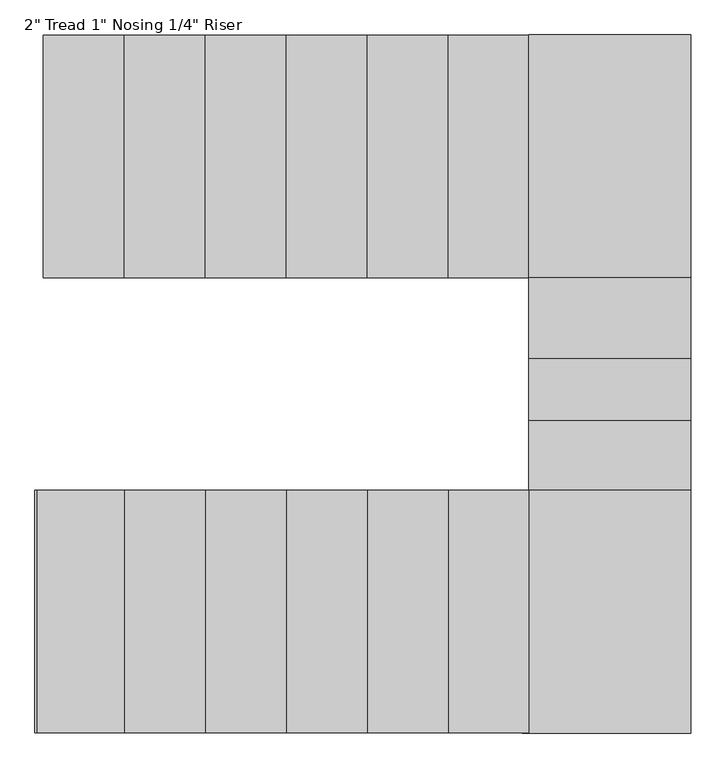
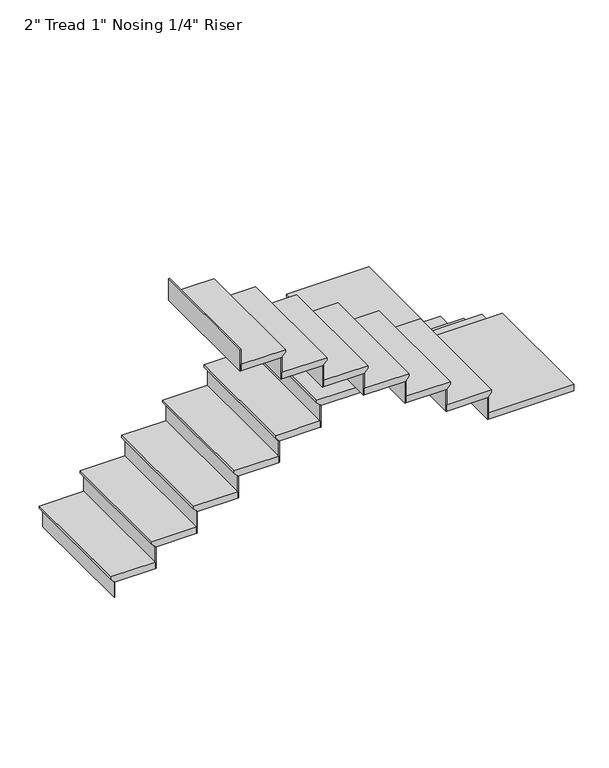
"""IFC4 building model written with IfcOpenShell, lengths in millimetres: stair flight geometry."""

from ifc_helpers import new_model, si_unit, origin, place, context, project, spatial, faceted_brep, source, transform, mapped, element, save


def stair_flight_95d2f6bb(model_context):
    return source(origin(), model_context, "Body", "Brep", [
        faceted_brep([(6477.0, 10054.8323212, 6246.2833333), (6477.0, 10054.8323212, 6265.3333333), (6477.0, 10969.2323212, 6265.3333333), (6477.0, 10969.2323212, 6246.2833333), (6502.4, 10054.8323212, 6220.8833333), (6502.4, 10969.2323212, 6220.8833333), (6807.2, 10054.8323212, 6265.3333333), (6807.2, 10969.2323212, 6265.3333333), (6502.4, 10969.2323212, 6214.5333333), (6807.2, 10969.2323212, 6214.5333333), (6807.2, 10054.8323212, 6214.5333333), (6502.4, 10054.8323212, 6214.5333333)], [[[0, 1, 2, 3]], [[4, 0, 3, 5]], [[2, 1, 6, 7]], [[8, 9, 10, 11]], [[2, 7, 9, 8, 5, 3]], [[8, 11, 4, 5]], [[6, 1, 0, 4, 11, 10]], [[7, 6, 10, 9]]]),
        faceted_brep([(6502.4, 10054.8323212, 6214.5333333), (6502.4, 10054.8323212, 6096.0), (6508.75, 10054.8323212, 6096.0), (6508.75, 10054.8323212, 6214.5333333), (6502.4, 10969.2323212, 6214.5333333), (6508.75, 10969.2323212, 6214.5333333), (6508.75, 10969.2323212, 6096.0), (6502.4, 10969.2323212, 6096.0)], [[[0, 1, 2, 3]], [[4, 5, 6, 7]], [[1, 0, 4, 7]], [[2, 1, 7, 6]], [[3, 2, 6, 5]], [[0, 3, 5, 4]]]),
        faceted_brep([(6807.2, 10054.8323212, 6383.8666667), (6807.2, 10054.8323212, 6214.5333333), (6813.55, 10054.8323212, 6214.5333333), (6813.55, 10054.8323212, 6383.8666667), (6807.2, 10969.2323212, 6383.8666667), (6813.55, 10969.2323212, 6383.8666667), (6813.55, 10969.2323212, 6214.5333333), (6807.2, 10969.2323212, 6214.5333333)], [[[0, 1, 2, 3]], [[4, 5, 6, 7]], [[1, 0, 4, 7]], [[2, 1, 7, 6]], [[3, 2, 6, 5]], [[0, 3, 5, 4]]]),
        faceted_brep([(6781.8, 10969.2323212, 6434.6666667), (6781.8, 10054.8323212, 6434.6666667), (7112.0, 10054.8323212, 6434.6666667), (7112.0, 10969.2323212, 6434.6666667), (6807.2, 10969.2323212, 6383.8666667), (7112.0, 10969.2323212, 6383.8666667), (7112.0, 10054.8323212, 6383.8666667), (6807.2, 10054.8323212, 6383.8666667), (6807.2, 10969.2323212, 6390.2166667), (6781.8, 10969.2323212, 6415.6166667), (6807.2, 10054.8323212, 6390.2166667), (6781.8, 10054.8323212, 6415.6166667)], [[[0, 1, 2, 3]], [[4, 5, 6, 7]], [[0, 3, 5, 4, 8, 9]], [[4, 7, 10, 8]], [[2, 1, 11, 10, 7, 6]], [[3, 2, 6, 5]], [[11, 1, 0, 9]], [[10, 11, 9, 8]]]),
        faceted_brep([(7112.0, 10054.8323212, 6553.2), (7112.0, 10054.8323212, 6383.8666667), (7118.35, 10054.8323212, 6383.8666667), (7118.35, 10054.8323212, 6553.2), (7112.0, 10969.2323212, 6553.2), (7118.35, 10969.2323212, 6553.2), (7118.35, 10969.2323212, 6383.8666667), (7112.0, 10969.2323212, 6383.8666667)], [[[0, 1, 2, 3]], [[4, 5, 6, 7]], [[1, 0, 4, 7]], [[2, 1, 7, 6]], [[3, 2, 6, 5]], [[0, 3, 5, 4]]]),
        faceted_brep([(7086.6, 10969.2323212, 6604.0), (7086.6, 10054.8323212, 6604.0), (7416.8, 10054.8323212, 6604.0), (7416.8, 10969.2323212, 6604.0), (7112.0, 10969.2323212, 6553.2), (7416.8, 10969.2323212, 6553.2), (7416.8, 10054.8323212, 6553.2), (7112.0, 10054.8323212, 6553.2), (7112.0, 10969.2323212, 6559.55), (7086.6, 10969.2323212, 6584.95), (7112.0, 10054.8323212, 6559.55), (7086.6, 10054.8323212, 6584.95)], [[[0, 1, 2, 3]], [[4, 5, 6, 7]], [[0, 3, 5, 4, 8, 9]], [[4, 7, 10, 8]], [[2, 1, 11, 10, 7, 6]], [[3, 2, 6, 5]], [[11, 1, 0, 9]], [[10, 11, 9, 8]]]),
        faceted_brep([(7416.8, 10054.8323212, 6722.5333333), (7416.8, 10054.8323212, 6553.2), (7423.15, 10054.8323212, 6553.2), (7423.15, 10054.8323212, 6722.5333333), (7416.8, 10969.2323212, 6722.5333333), (7423.15, 10969.2323212, 6722.5333333), (7423.15, 10969.2323212, 6553.2), (7416.8, 10969.2323212, 6553.2)], [[[0, 1, 2, 3]], [[4, 5, 6, 7]], [[1, 0, 4, 7]], [[2, 1, 7, 6]], [[3, 2, 6, 5]], [[0, 3, 5, 4]]]),
        faceted_brep([(7391.4, 10969.2323212, 6773.3333333), (7391.4, 10054.8323212, 6773.3333333), (7721.6, 10054.8323212, 6773.3333333), (7721.6, 10969.2323212, 6773.3333333), (7416.8, 10969.2323212, 6722.5333333), (7721.6, 10969.2323212, 6722.5333333), (7721.6, 10054.8323212, 6722.5333333), (7416.8, 10054.8323212, 6722.5333333), (7416.8, 10969.2323212, 6728.8833333), (7391.4, 10969.2323212, 6754.2833333), (7416.8, 10054.8323212, 6728.8833333), (7391.4, 10054.8323212, 6754.2833333)], [[[0, 1, 2, 3]], [[4, 5, 6, 7]], [[0, 3, 5, 4, 8, 9]], [[4, 7, 10, 8]], [[2, 1, 11, 10, 7, 6]], [[3, 2, 6, 5]], [[11, 1, 0, 9]], [[10, 11, 9, 8]]]),
        faceted_brep([(7721.6, 10054.8323212, 6891.8666667), (7721.6, 10054.8323212, 6722.5333333), (7727.95, 10054.8323212, 6722.5333333), (7727.95, 10054.8323212, 6891.8666667), (7721.6, 10969.2323212, 6891.8666667), (7727.95, 10969.2323212, 6891.8666667), (7727.95, 10969.2323212, 6722.5333333), (7721.6, 10969.2323212, 6722.5333333)], [[[0, 1, 2, 3]], [[4, 5, 6, 7]], [[1, 0, 4, 7]], [[2, 1, 7, 6]], [[3, 2, 6, 5]], [[0, 3, 5, 4]]]),
        faceted_brep([(7696.2, 10969.2323212, 6942.6666667), (7696.2, 10054.8323212, 6942.6666667), (8026.4, 10054.8323212, 6942.6666667), (8026.4, 10969.2323212, 6942.6666667), (7721.6, 10969.2323212, 6891.8666667), (8026.4, 10969.2323212, 6891.8666667), (8026.4, 10054.8323212, 6891.8666667), (7721.6, 10054.8323212, 6891.8666667), (7721.6, 10969.2323212, 6898.2166667), (7696.2, 10969.2323212, 6923.6166667), (7721.6, 10054.8323212, 6898.2166667), (7696.2, 10054.8323212, 6923.6166667)], [[[0, 1, 2, 3]], [[4, 5, 6, 7]], [[0, 3, 5, 4, 8, 9]], [[4, 7, 10, 8]], [[2, 1, 11, 10, 7, 6]], [[3, 2, 6, 5]], [[11, 1, 0, 9]], [[10, 11, 9, 8]]]),
        faceted_brep([(8026.4, 10054.8323212, 7061.2), (8026.4, 10054.8323212, 6891.8666667), (8032.75, 10054.8323212, 6891.8666667), (8032.75, 10054.8323212, 7061.2), (8026.4, 10969.2323212, 7061.2), (8032.75, 10969.2323212, 7061.2), (8032.75, 10969.2323212, 6891.8666667), (8026.4, 10969.2323212, 6891.8666667)], [[[0, 1, 2, 3]], [[4, 5, 6, 7]], [[1, 0, 4, 7]], [[2, 1, 7, 6]], [[3, 2, 6, 5]], [[0, 3, 5, 4]]]),
        faceted_brep([(8001.0, 10969.2323212, 7112.0), (8001.0, 10054.8323212, 7112.0), (8331.2, 10054.8323212, 7112.0), (8331.2, 10969.2323212, 7112.0), (8026.4, 10969.2323212, 7061.2), (8331.2, 10969.2323212, 7061.2), (8331.2, 10054.8323212, 7061.2), (8026.4, 10054.8323212, 7061.2), (8026.4, 10969.2323212, 7067.55), (8001.0, 10969.2323212, 7092.95), (8026.4, 10054.8323212, 7067.55), (8001.0, 10054.8323212, 7092.95)], [[[0, 1, 2, 3]], [[4, 5, 6, 7]], [[0, 3, 5, 4, 8, 9]], [[4, 7, 10, 8]], [[2, 1, 11, 10, 7, 6]], [[3, 2, 6, 5]], [[11, 1, 0, 9]], [[10, 11, 9, 8]]]),
        faceted_brep([(8331.2, 10054.8323212, 7230.5333333), (8331.2, 10054.8323212, 7061.2), (8337.55, 10054.8323212, 7061.2), (8337.55, 10054.8323212, 7230.5333333), (8331.2, 10969.2323212, 7230.5333333), (8337.55, 10969.2323212, 7230.5333333), (8337.55, 10969.2323212, 7061.2), (8331.2, 10969.2323212, 7061.2)], [[[0, 1, 2, 3]], [[4, 5, 6, 7]], [[1, 0, 4, 7]], [[2, 1, 7, 6]], [[3, 2, 6, 5]], [[0, 3, 5, 4]]]),
        faceted_brep([(8915.4, 10029.4323212, 7281.3333333), (8915.4, 10969.2323212, 7281.3333333), (8305.8, 10969.2323212, 7281.3333333), (8305.8, 10029.4323212, 7281.3333333), (8915.4, 10969.2323212, 7230.5333333), (8915.4, 10029.4323212, 7230.5333333), (8305.8, 10029.4323212, 7230.5333333), (8305.8, 10054.8323212, 7230.5333333), (8331.2, 10054.8323212, 7230.5333333), (8331.2, 10969.2323212, 7230.5333333), (8331.2, 10969.2323212, 7236.8833333), (8305.8, 10969.2323212, 7262.2833333), (8331.2, 10054.8323212, 7236.8833333), (8305.8, 10054.8323212, 7262.2833333)], [[[0, 1, 2, 3]], [[4, 5, 6, 7, 8, 9]], [[1, 0, 5, 4]], [[2, 1, 4, 9, 10, 11]], [[9, 8, 12, 10]], [[8, 7, 13, 12]], [[3, 2, 11, 13, 7, 6]], [[0, 3, 6, 5]], [[11, 10, 12, 13]]]),
        faceted_brep([(8305.8, 10029.4323212, 7399.8666667), (8305.8, 10029.4323212, 7230.5333333), (8305.8, 10023.0823212, 7230.5333333), (8305.8, 10023.0823212, 7399.8666667), (8915.4, 10029.4323212, 7399.8666667), (8915.4, 10023.0823212, 7399.8666667), (8915.4, 10023.0823212, 7230.5333333), (8915.4, 10029.4323212, 7230.5333333)], [[[0, 1, 2, 3]], [[4, 5, 6, 7]], [[1, 0, 4, 7]], [[2, 1, 7, 6]], [[3, 2, 6, 5]], [[0, 3, 5, 4]]]),
        faceted_brep([(8915.4, 10054.8323212, 7450.6666667), (8305.8, 10054.8323212, 7450.6666667), (8305.8, 9724.6323212, 7450.6666667), (8915.4, 9724.6323212, 7450.6666667), (8915.4, 10029.4323212, 7399.8666667), (8915.4, 9724.6323212, 7399.8666667), (8305.8, 9724.6323212, 7399.8666667), (8305.8, 10029.4323212, 7399.8666667), (8915.4, 10029.4323212, 7406.2166667), (8915.4, 10054.8323212, 7431.6166667), (8305.8, 10029.4323212, 7406.2166667), (8305.8, 10054.8323212, 7431.6166667)], [[[0, 1, 2, 3]], [[4, 5, 6, 7]], [[0, 3, 5, 4, 8, 9]], [[4, 7, 10, 8]], [[2, 1, 11, 10, 7, 6]], [[3, 2, 6, 5]], [[11, 1, 0, 9]], [[10, 11, 9, 8]]]),
        faceted_brep([(8305.8, 9724.6323212, 7569.2), (8305.8, 9724.6323212, 7399.8666667), (8305.8, 9718.2823212, 7399.8666667), (8305.8, 9718.2823212, 7569.2), (8915.4, 9724.6323212, 7569.2), (8915.4, 9718.2823212, 7569.2), (8915.4, 9718.2823212, 7399.8666667), (8915.4, 9724.6323212, 7399.8666667)], [[[0, 1, 2, 3]], [[4, 5, 6, 7]], [[1, 0, 4, 7]], [[2, 1, 7, 6]], [[3, 2, 6, 5]], [[0, 3, 5, 4]]]),
        faceted_brep([(8915.4, 9750.0323212, 7620.0), (8305.8, 9750.0323212, 7620.0), (8305.8, 9491.8832929, 7620.0), (8915.4, 9491.8832929, 7620.0), (8915.4, 9724.6323212, 7569.2), (8915.4, 9491.8832929, 7569.2), (8305.8, 9491.8832929, 7569.2), (8305.8, 9724.6323212, 7569.2), (8915.4, 9724.6323212, 7575.55), (8915.4, 9750.0323212, 7600.95), (8305.8, 9724.6323212, 7575.55), (8305.8, 9750.0323212, 7600.95)], [[[0, 1, 2, 3]], [[4, 5, 6, 7]], [[0, 3, 5, 4, 8, 9]], [[4, 7, 10, 8]], [[2, 1, 11, 10, 7, 6]], [[3, 2, 6, 5]], [[11, 1, 0, 9]], [[10, 11, 9, 8]]]),
        faceted_brep([(8305.8, 9491.8832929, 7738.5333333), (8305.8, 9491.8832929, 7569.2), (8305.8, 9485.5332929, 7569.2), (8305.8, 9485.5332929, 7738.5333333), (8915.4, 9491.8832929, 7738.5333333), (8915.4, 9485.5332929, 7738.5333333), (8915.4, 9485.5332929, 7569.2), (8915.4, 9491.8832929, 7569.2)], [[[0, 1, 2, 3]], [[4, 5, 6, 7]], [[1, 0, 4, 7]], [[2, 1, 7, 6]], [[3, 2, 6, 5]], [[0, 3, 5, 4]]]),
        faceted_brep([(8915.4, 9517.2832929, 7789.3333333), (8305.8, 9517.2832929, 7789.3333333), (8305.8, 9229.3323212, 7789.3333333), (8915.4, 9229.3323212, 7789.3333333), (8915.4, 9491.8832929, 7738.5333333), (8915.4, 9229.3323212, 7738.5333333), (8305.8, 9229.3323212, 7738.5333333), (8305.8, 9491.8832929, 7738.5333333), (8915.4, 9491.8832929, 7744.8833333), (8915.4, 9517.2832929, 7770.2833333), (8305.8, 9491.8832929, 7744.8833333), (8305.8, 9517.2832929, 7770.2833333)], [[[0, 1, 2, 3]], [[4, 5, 6, 7]], [[0, 3, 5, 4, 8, 9]], [[4, 7, 10, 8]], [[2, 1, 11, 10, 7, 6]], [[3, 2, 6, 5]], [[11, 1, 0, 9]], [[10, 11, 9, 8]]]),
        faceted_brep([(8305.8, 9229.3323212, 7907.8666667), (8305.8, 9229.3323212, 7738.5333333), (8305.8, 9222.9823212, 7738.5333333), (8305.8, 9222.9823212, 7907.8666667), (8915.4, 9229.3323212, 7907.8666667), (8915.4, 9222.9823212, 7907.8666667), (8915.4, 9222.9823212, 7738.5333333), (8915.4, 9229.3323212, 7738.5333333)], [[[0, 1, 2, 3]], [[4, 5, 6, 7]], [[1, 0, 4, 7]], [[2, 1, 7, 6]], [[3, 2, 6, 5]], [[0, 3, 5, 4]]]),
        faceted_brep([(8280.4, 8340.3323212, 7958.6666667), (8915.4, 8340.3323212, 7958.6666667), (8915.4, 9254.7323212, 7958.6666667), (8280.4, 9254.7323212, 7958.6666667), (8915.4, 8340.3323212, 7907.8666667), (8280.4, 8340.3323212, 7907.8666667), (8280.4, 9254.7323212, 7907.8666667), (8305.8, 9254.7323212, 7907.8666667), (8305.8, 9229.3323212, 7907.8666667), (8915.4, 9229.3323212, 7907.8666667), (8915.4, 9229.3323212, 7914.2166667), (8915.4, 9254.7323212, 7939.6166667), (8305.8, 9229.3323212, 7914.2166667), (8305.8, 9254.7323212, 7939.6166667)], [[[0, 1, 2, 3]], [[4, 5, 6, 7, 8, 9]], [[1, 0, 5, 4]], [[2, 1, 4, 9, 10, 11]], [[9, 8, 12, 10]], [[8, 7, 13, 12]], [[3, 2, 11, 13, 7, 6]], [[0, 3, 6, 5]], [[11, 10, 12, 13]]]),
        faceted_brep([(8280.4, 9254.7323212, 8077.2), (8280.4, 9254.7323212, 7907.8666667), (8274.05, 9254.7323212, 7907.8666667), (8274.05, 9254.7323212, 8077.2), (8280.4, 8340.3323212, 8077.2), (8274.05, 8340.3323212, 8077.2), (8274.05, 8340.3323212, 7907.8666667), (8280.4, 8340.3323212, 7907.8666667)], [[[0, 1, 2, 3]], [[4, 5, 6, 7]], [[1, 0, 4, 7]], [[2, 1, 7, 6]], [[3, 2, 6, 5]], [[0, 3, 5, 4]]]),
        faceted_brep([(8305.8, 8340.3323212, 8128.0), (8305.8, 9254.7323212, 8128.0), (7975.6, 9254.7323212, 8128.0), (7975.6, 8340.3323212, 8128.0), (8280.4, 8340.3323212, 8077.2), (7975.6, 8340.3323212, 8077.2), (7975.6, 9254.7323212, 8077.2), (8280.4, 9254.7323212, 8077.2), (8280.4, 8340.3323212, 8083.55), (8305.8, 8340.3323212, 8108.95), (8280.4, 9254.7323212, 8083.55), (8305.8, 9254.7323212, 8108.95)], [[[0, 1, 2, 3]], [[4, 5, 6, 7]], [[0, 3, 5, 4, 8, 9]], [[4, 7, 10, 8]], [[2, 1, 11, 10, 7, 6]], [[3, 2, 6, 5]], [[11, 1, 0, 9]], [[10, 11, 9, 8]]]),
        faceted_brep([(7975.6, 9254.7323212, 8246.5333333), (7975.6, 9254.7323212, 8077.2), (7969.25, 9254.7323212, 8077.2), (7969.25, 9254.7323212, 8246.5333333), (7975.6, 8340.3323212, 8246.5333333), (7969.25, 8340.3323212, 8246.5333333), (7969.25, 8340.3323212, 8077.2), (7975.6, 8340.3323212, 8077.2)], [[[0, 1, 2, 3]], [[4, 5, 6, 7]], [[1, 0, 4, 7]], [[2, 1, 7, 6]], [[3, 2, 6, 5]], [[0, 3, 5, 4]]]),
        faceted_brep([(8001.0, 8340.3323212, 8297.3333333), (8001.0, 9254.7323212, 8297.3333333), (7670.8, 9254.7323212, 8297.3333333), (7670.8, 8340.3323212, 8297.3333333), (7975.6, 8340.3323212, 8246.5333333), (7670.8, 8340.3323212, 8246.5333333), (7670.8, 9254.7323212, 8246.5333333), (7975.6, 9254.7323212, 8246.5333333), (7975.6, 8340.3323212, 8252.8833333), (8001.0, 8340.3323212, 8278.2833333), (7975.6, 9254.7323212, 8252.8833333), (8001.0, 9254.7323212, 8278.2833333)], [[[0, 1, 2, 3]], [[4, 5, 6, 7]], [[0, 3, 5, 4, 8, 9]], [[4, 7, 10, 8]], [[2, 1, 11, 10, 7, 6]], [[3, 2, 6, 5]], [[11, 1, 0, 9]], [[10, 11, 9, 8]]]),
        faceted_brep([(7670.8, 9254.7323212, 8415.8666667), (7670.8, 9254.7323212, 8246.5333333), (7664.45, 9254.7323212, 8246.5333333), (7664.45, 9254.7323212, 8415.8666667), (7670.8, 8340.3323212, 8415.8666667), (7664.45, 8340.3323212, 8415.8666667), (7664.45, 8340.3323212, 8246.5333333), (7670.8, 8340.3323212, 8246.5333333)], [[[0, 1, 2, 3]], [[4, 5, 6, 7]], [[1, 0, 4, 7]], [[2, 1, 7, 6]], [[3, 2, 6, 5]], [[0, 3, 5, 4]]]),
        faceted_brep([(7696.2, 8340.3323212, 8466.6666667), (7696.2, 9254.7323212, 8466.6666667), (7366.0, 9254.7323212, 8466.6666667), (7366.0, 8340.3323212, 8466.6666667), (7670.8, 8340.3323212, 8415.8666667), (7366.0, 8340.3323212, 8415.8666667), (7366.0, 9254.7323212, 8415.8666667), (7670.8, 9254.7323212, 8415.8666667), (7670.8, 8340.3323212, 8422.2166667), (7696.2, 8340.3323212, 8447.6166667), (7670.8, 9254.7323212, 8422.2166667), (7696.2, 9254.7323212, 8447.6166667)], [[[0, 1, 2, 3]], [[4, 5, 6, 7]], [[0, 3, 5, 4, 8, 9]], [[4, 7, 10, 8]], [[2, 1, 11, 10, 7, 6]], [[3, 2, 6, 5]], [[11, 1, 0, 9]], [[10, 11, 9, 8]]]),
        faceted_brep([(7366.0, 9254.7323212, 8585.2), (7366.0, 9254.7323212, 8415.8666667), (7359.65, 9254.7323212, 8415.8666667), (7359.65, 9254.7323212, 8585.2), (7366.0, 8340.3323212, 8585.2), (7359.65, 8340.3323212, 8585.2), (7359.65, 8340.3323212, 8415.8666667), (7366.0, 8340.3323212, 8415.8666667)], [[[0, 1, 2, 3]], [[4, 5, 6, 7]], [[1, 0, 4, 7]], [[2, 1, 7, 6]], [[3, 2, 6, 5]], [[0, 3, 5, 4]]]),
        faceted_brep([(7391.4, 8340.3323212, 8636.0), (7391.4, 9254.7323212, 8636.0), (7061.2, 9254.7323212, 8636.0), (7061.2, 8340.3323212, 8636.0), (7366.0, 8340.3323212, 8585.2), (7061.2, 8340.3323212, 8585.2), (7061.2, 9254.7323212, 8585.2), (7366.0, 9254.7323212, 8585.2), (7366.0, 8340.3323212, 8591.55), (7391.4, 8340.3323212, 8616.95), (7366.0, 9254.7323212, 8591.55), (7391.4, 9254.7323212, 8616.95)], [[[0, 1, 2, 3]], [[4, 5, 6, 7]], [[0, 3, 5, 4, 8, 9]], [[4, 7, 10, 8]], [[2, 1, 11, 10, 7, 6]], [[3, 2, 6, 5]], [[11, 1, 0, 9]], [[10, 11, 9, 8]]]),
        faceted_brep([(7061.2, 9254.7323212, 8754.5333333), (7061.2, 9254.7323212, 8585.2), (7054.85, 9254.7323212, 8585.2), (7054.85, 9254.7323212, 8754.5333333), (7061.2, 8340.3323212, 8754.5333333), (7054.85, 8340.3323212, 8754.5333333), (7054.85, 8340.3323212, 8585.2), (7061.2, 8340.3323212, 8585.2)], [[[0, 1, 2, 3]], [[4, 5, 6, 7]], [[1, 0, 4, 7]], [[2, 1, 7, 6]], [[3, 2, 6, 5]], [[0, 3, 5, 4]]]),
        faceted_brep([(7086.6, 8340.3323212, 8805.3333333), (7086.6, 9254.7323212, 8805.3333333), (6756.4, 9254.7323212, 8805.3333333), (6756.4, 8340.3323212, 8805.3333333), (7061.2, 8340.3323212, 8754.5333333), (6756.4, 8340.3323212, 8754.5333333), (6756.4, 9254.7323212, 8754.5333333), (7061.2, 9254.7323212, 8754.5333333), (7061.2, 8340.3323212, 8760.8833333), (7086.6, 8340.3323212, 8786.2833333), (7061.2, 9254.7323212, 8760.8833333), (7086.6, 9254.7323212, 8786.2833333)], [[[0, 1, 2, 3]], [[4, 5, 6, 7]], [[0, 3, 5, 4, 8, 9]], [[4, 7, 10, 8]], [[2, 1, 11, 10, 7, 6]], [[3, 2, 6, 5]], [[11, 1, 0, 9]], [[10, 11, 9, 8]]]),
        faceted_brep([(6756.4, 9254.7323212, 8923.8666667), (6756.4, 9254.7323212, 8754.5333333), (6750.05, 9254.7323212, 8754.5333333), (6750.05, 9254.7323212, 8923.8666667), (6756.4, 8340.3323212, 8923.8666667), (6750.05, 8340.3323212, 8923.8666667), (6750.05, 8340.3323212, 8754.5333333), (6756.4, 8340.3323212, 8754.5333333)], [[[0, 1, 2, 3]], [[4, 5, 6, 7]], [[1, 0, 4, 7]], [[2, 1, 7, 6]], [[3, 2, 6, 5]], [[0, 3, 5, 4]]]),
        faceted_brep([(6451.6, 9254.7323212, 9093.2), (6451.6, 9254.7323212, 8923.8666667), (6445.25, 9254.7323212, 8923.8666667), (6445.25, 9254.7323212, 9093.2), (6451.6, 8340.3323212, 9093.2), (6445.25, 8340.3323212, 9093.2), (6445.25, 8340.3323212, 8923.8666667), (6451.6, 8340.3323212, 8923.8666667)], [[[0, 1, 2, 3]], [[4, 5, 6, 7]], [[1, 0, 4, 7]], [[2, 1, 7, 6]], [[3, 2, 6, 5]], [[0, 3, 5, 4]]]),
        faceted_brep([(6781.8, 8340.3323212, 8974.6666667), (6781.8, 9254.7323212, 8974.6666667), (6451.6, 9254.7323212, 8974.6666667), (6451.6, 8340.3323212, 8974.6666667), (6756.4, 8340.3323212, 8923.8666667), (6451.6, 8340.3323212, 8923.8666667), (6451.6, 9254.7323212, 8923.8666667), (6756.4, 9254.7323212, 8923.8666667), (6756.4, 8340.3323212, 8930.2166667), (6781.8, 8340.3323212, 8955.6166667), (6756.4, 9254.7323212, 8930.2166667), (6781.8, 9254.7323212, 8955.6166667)], [[[0, 1, 2, 3]], [[4, 5, 6, 7]], [[0, 3, 5, 4, 8, 9]], [[4, 7, 10, 8]], [[2, 1, 11, 10, 7, 6]], [[3, 2, 6, 5]], [[11, 1, 0, 9]], [[10, 11, 9, 8]]]),
    ])


if __name__ == "__main__":
    model = new_model("IFC4")
    model_context = context("Model", 3, world=origin())
    ifc_project = project(units=[si_unit("LENGTHUNIT", "METRE", prefix="MILLI")], contexts=[model_context])
    site = spatial("IfcSite", under=ifc_project)
    building = spatial("IfcBuilding", under=site)
    placement = place(None, origin())
    stair_flight_shape = stair_flight_95d2f6bb(model_context)
    element("IfcStairFlight", 1, ObjectType="2\" Tread 1\" Nosing 1/4\" Riser", at=placement, inside=building, context=model_context, shape_type="MappedRepresentation", body=[
        mapped(stair_flight_shape, transform((0.0, 0.0, 0.0), x_axis=(1.0, 0.0, 0.0), y_axis=(0.0, 1.0, 0.0), z_axis=(0.0, 0.0, 1.0))),
    ])
    save(model, "model.ifc")
